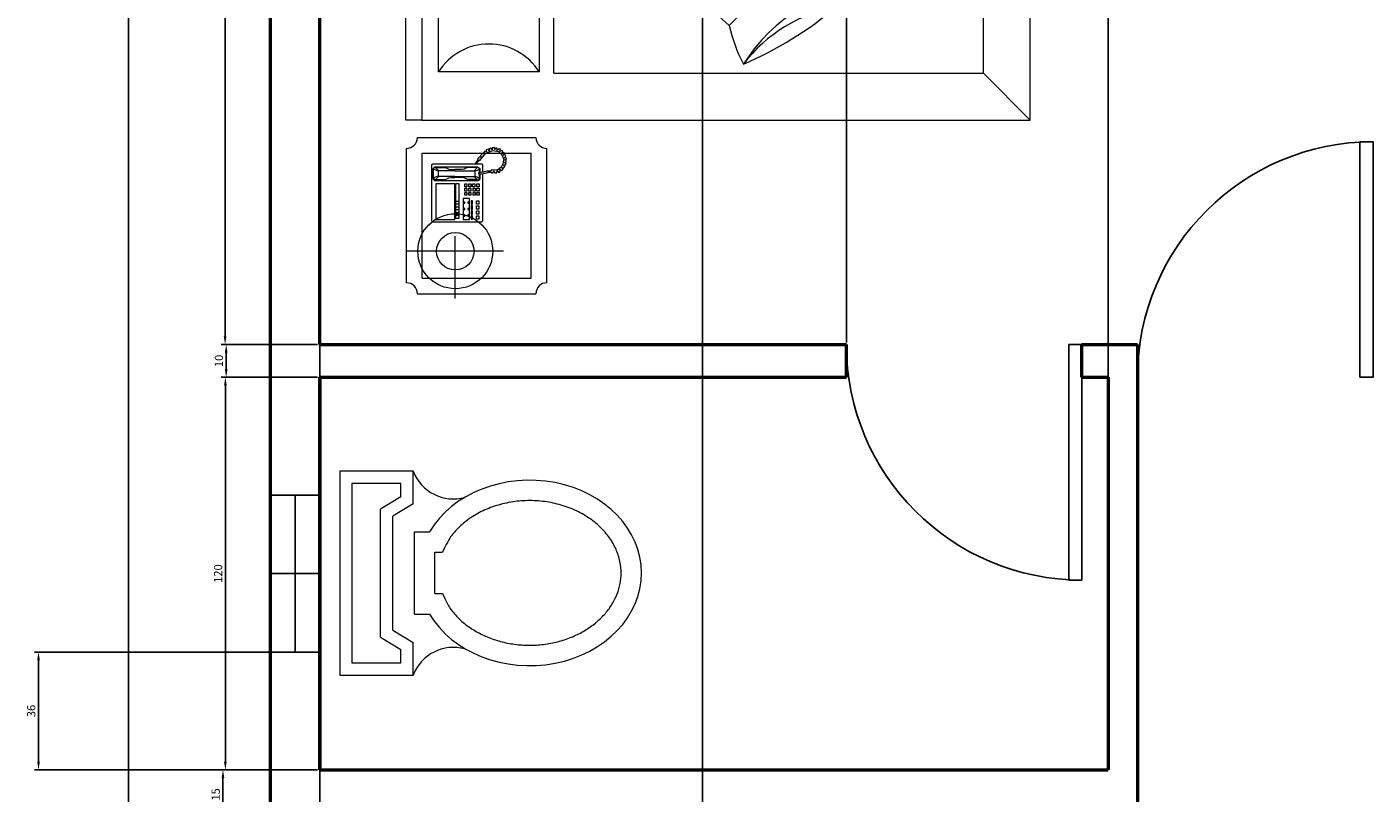
# Model space of a CAD drawing. Units: inches. Extents: x 604 to 3492, y -123 to 1737.
# Tile 13 of 20: x 1500 to 1912, y 836 to 1070. Entities that reach past the tile are written whole.
import ezdxf

# ---------------------------------------------------------------- set-up
doc = ezdxf.new("R2010")
doc.units = ezdxf.units.IN
for name, color, linetype, lineweight in [('A-ANNO-DIMS', 2, 'Continuous', 18), ('A-DOOR', 3, 'Continuous', 25), ('A-FLOR-FIXT', 9, 'Continuous', 18), ('A-FURN', 8, 'Continuous', 18), ('A-GLAZ', 4, 'Continuous', 25), ('A-WALL', 7, 'Continuous', 50)]:
    doc.layers.add(name, color=color, linetype=linetype, lineweight=lineweight)
doc.styles.get("Standard").update_dxf_attribs({"font": 'arial.ttf'})
doc.dimstyles.new('ISO-25', dxfattribs={"dimtxt": 2.5, "dimasz": 2.5, "dimexe": 1.25, "dimexo": 0.625, "dimtad": 1, "dimtxsty": 'Standard', "dimcen": 2.5, "dimadec": 0, "dimazin": 0, "dimtfac": 1, "dimtmove": 0, "dimatfit": 3, "dimfxl": 1, "dimarcsym": 0})

# ---------------------------------------------------------------- blocks, each defined once
blk = doc.blocks.new('A$C50B66110')
for p, q in [((0.0503, 1.9981), (0.4803, 1.9981)), ((0.1513, 1.6871), (0.1513, 1.9967)), ((0.5716, 1.9488), (0.5716, 2)), ((0.5716, 2), (2.0719, 2)), ((2.0719, 1.9488), (2.0719, 2)), ((2.5701, 1.9993), (2.1401, 1.9993)), ((0.0153, 1.9631), (0.0153, 1.5831)), ((0.0653, 1.9481), (0.0653, 1.5981)), ((0.0653, 1.9481), (0.4653, 1.9481)), ((0.4653, 1.9481), (0.4653, 1.5981)), ((0.5153, 1.9631), (0.5153, 1.5831)), ((2.0719, 1.9488), (0.5716, 1.9488)), ((0.5716, 1.9488), (0.5716, 0)), ((2.0719, 0), (2.0719, 1.9488)), ((2.1051, 1.9643), (2.1051, 1.5843)), ((2.1551, 1.9493), (2.1551, 1.5993)), ((2.5551, 1.9493), (2.1551, 1.9493)), ((2.5551, 1.9493), (2.5551, 1.5993)), ((2.6051, 1.9643), (2.6051, 1.5843)), ((2.3505, 1.62), (2.3505, 1.9295)), ((0.7257, 1.5725), (0.7257, 1.8954)), ((0.7257, 1.8954), (1.2113, 1.8954)), ((1.2113, 1.8954), (1.2113, 1.5725)), ((1.4007, 1.5725), (1.4007, 1.8954)), ((1.4007, 1.8954), (1.8863, 1.8954)), ((1.8863, 1.8954), (1.8863, 1.5725)), ((0, 1.8416), (0.2001, 1.8416)), ((2.5018, 1.7744), (2.2017, 1.7744)), ((0.0653, 1.5981), (0.4653, 1.5981)), ((2.5551, 1.5993), (2.1551, 1.5993)), ((1.2113, 1.5725), (0.7257, 1.5725)), ((1.8863, 1.5725), (1.4007, 1.5725)), ((0.0503, 1.5481), (0.4803, 1.5481)), ((1.5665, 1.5254), (1.5665, 1.0802)), ((1.5665, 1.5254), (1.9219, 1.0802)), ((2.5701, 1.5493), (2.1401, 1.5493)), ((1.9219, 1.0802), (1.5665, 1.0802)), ((0.5716, 0), (0.7216, 0.15)), ((2.0719, 0), (1.9219, 0.15)), ((0.5716, 0), (2.0719, 0))]:
    blk.add_line(p, q)
at = {"linetype": 'ByBlock'}
for p, q in [((0.2481, 1.9162), (0.2458, 1.9139)), ((0.2458, 1.9139), (0.2458, 1.7562)), ((0.2481, 1.9162), (0.4287, 1.9162)), ((0.2526, 1.9036), (0.2526, 1.8431)), ((0.3669, 1.9036), (0.2526, 1.9036)), ((0.3669, 1.8431), (0.3669, 1.9036)), ((0.3772, 1.9071), (0.3818, 1.9128)), ((0.3772, 1.7688), (0.3772, 1.9071)), ((0.3818, 1.9094), (0.3807, 1.9048)), ((0.3807, 1.9048), (0.3807, 1.8739)), ((0.3807, 1.9048), (0.3909, 1.8945)), ((0.3818, 1.9128), (0.4161, 1.9128)), ((0.3864, 1.9116), (0.3818, 1.9094)), ((0.3921, 1.8968), (0.3864, 1.9116)), ((0.3864, 1.9116), (0.4138, 1.9116)), ((0.4081, 1.8968), (0.4138, 1.9116)), ((0.4195, 1.9048), (0.4092, 1.8945)), ((0.4138, 1.9116), (0.4184, 1.9094)), ((0.4161, 1.9128), (0.4218, 1.9071)), ((0.4184, 1.9094), (0.4195, 1.9048)), ((0.4195, 1.9048), (0.4195, 1.8739)), ((0.4218, 1.9071), (0.4218, 1.7699)), ((0.4287, 1.9162), (0.4309, 1.9139)), ((0.4309, 1.9139), (0.4309, 1.7562)), ((0.3807, 1.8739), (0.3829, 1.8682)), ((0.3829, 1.8682), (0.3864, 1.8625)), ((0.3864, 1.8625), (0.3875, 1.8545)), ((0.3875, 1.8545), (0.3875, 1.8431)), ((0.3909, 1.8945), (0.3921, 1.8968)), ((0.3909, 1.8431), (0.3909, 1.8945)), ((0.4081, 1.8968), (0.3921, 1.8968)), ((0.4092, 1.8945), (0.4081, 1.8968)), ((0.4092, 1.8431), (0.4092, 1.8945)), ((0.4138, 1.8625), (0.4127, 1.8545)), ((0.4127, 1.8545), (0.4127, 1.8431)), ((0.4172, 1.8682), (0.4138, 1.8625)), ((0.4195, 1.8739), (0.4172, 1.8682)), ((0.2526, 1.8431), (0.3669, 1.8431)), ((0.3201, 1.8168), (0.2526, 1.8168)), ((0.2526, 1.8168), (0.2526, 1.7962)), ((0.2572, 1.8408), (0.2572, 1.8294)), ((0.3669, 1.8408), (0.2572, 1.8408)), ((0.2572, 1.8294), (0.3669, 1.8294)), ((0.2675, 1.8145), (0.2641, 1.8145)), ((0.2641, 1.8145), (0.2641, 1.8111)), ((0.2641, 1.8111), (0.2675, 1.8111)), ((0.2664, 1.8408), (0.2664, 1.8294)), ((0.2675, 1.8111), (0.2675, 1.8145)), ((0.2755, 1.8408), (0.2755, 1.8294)), ((0.2846, 1.8408), (0.2846, 1.8294)), ((0.2846, 1.8145), (0.2846, 1.8111)), ((0.2881, 1.8145), (0.2846, 1.8145)), ((0.2846, 1.8111), (0.2881, 1.8111)), ((0.2881, 1.8111), (0.2881, 1.8145)), ((0.2938, 1.8408), (0.2938, 1.8294)), ((0.3029, 1.8408), (0.3029, 1.8294)), ((0.3052, 1.8145), (0.3052, 1.8111)), ((0.3086, 1.8145), (0.3052, 1.8145)), ((0.3052, 1.8111), (0.3086, 1.8111)), ((0.3086, 1.8111), (0.3086, 1.8145)), ((0.3121, 1.8408), (0.3121, 1.8294)), ((0.3201, 1.7962), (0.3201, 1.8168)), ((0.3304, 1.8111), (0.3395, 1.8111)), ((0.3304, 1.8042), (0.3304, 1.8111)), ((0.3395, 1.8111), (0.3395, 1.8042)), ((0.3441, 1.8042), (0.3441, 1.8111)), ((0.3441, 1.8111), (0.3532, 1.8111)), ((0.3532, 1.8111), (0.3532, 1.8042)), ((0.3578, 1.8111), (0.3669, 1.8111)), ((0.3578, 1.8042), (0.3578, 1.8111)), ((0.3669, 1.8294), (0.3669, 1.8408)), ((0.3669, 1.8111), (0.3669, 1.8042)), ((0.3829, 1.8076), (0.3864, 1.8134)), ((0.3864, 1.8134), (0.3875, 1.8214)), ((0.3875, 1.8214), (0.3875, 1.8431)), ((0.3909, 1.8431), (0.3909, 1.7813)), ((0.4092, 1.8431), (0.4092, 1.7813)), ((0.4127, 1.8214), (0.4127, 1.8431)), ((0.4138, 1.8134), (0.4127, 1.8214)), ((0.4172, 1.8076), (0.4138, 1.8134)), ((0.2526, 1.7962), (0.3201, 1.7962)), ((0.2652, 1.7905), (0.2538, 1.7905)), ((0.2538, 1.7905), (0.2538, 1.7859)), ((0.2538, 1.7859), (0.2652, 1.7859)), ((0.2538, 1.7665), (0.2538, 1.7733)), ((0.2538, 1.7733), (0.2652, 1.7733)), ((0.2641, 1.8019), (0.2641, 1.7985)), ((0.2675, 1.8019), (0.2641, 1.8019)), ((0.2641, 1.7985), (0.2675, 1.7985)), ((0.2652, 1.7859), (0.2652, 1.7905)), ((0.2652, 1.7733), (0.2652, 1.7665)), ((0.2675, 1.7985), (0.2675, 1.8019)), ((0.2812, 1.7905), (0.2698, 1.7905)), ((0.2698, 1.7905), (0.2698, 1.7859)), ((0.2698, 1.7859), (0.2812, 1.7859)), ((0.2698, 1.7665), (0.2698, 1.7733)), ((0.2698, 1.7733), (0.2812, 1.7733)), ((0.2812, 1.7859), (0.2812, 1.7905)), ((0.2812, 1.7733), (0.2812, 1.7665)), ((0.2846, 1.8019), (0.2846, 1.7985)), ((0.2881, 1.8019), (0.2846, 1.8019)), ((0.2846, 1.7985), (0.2881, 1.7985)), ((0.2972, 1.7905), (0.2858, 1.7905)), ((0.2858, 1.7905), (0.2858, 1.7859)), ((0.2858, 1.7859), (0.2972, 1.7859)), ((0.2858, 1.7665), (0.2858, 1.7733)), ((0.2858, 1.7733), (0.2972, 1.7733)), ((0.2881, 1.7985), (0.2881, 1.8019)), ((0.2972, 1.7859), (0.2972, 1.7905)), ((0.2972, 1.7733), (0.2972, 1.7665)), ((0.3018, 1.7905), (0.3018, 1.7859)), ((0.3132, 1.7905), (0.3018, 1.7905)), ((0.3018, 1.7859), (0.3132, 1.7859)), ((0.3018, 1.7733), (0.3132, 1.7733)), ((0.3018, 1.7665), (0.3018, 1.7733)), ((0.3052, 1.8019), (0.3052, 1.7985)), ((0.3086, 1.8019), (0.3052, 1.8019)), ((0.3052, 1.7985), (0.3086, 1.7985)), ((0.3086, 1.7985), (0.3086, 1.8019)), ((0.3132, 1.7859), (0.3132, 1.7905)), ((0.3132, 1.7733), (0.3132, 1.7665)), ((0.3395, 1.8042), (0.3304, 1.8042)), ((0.3304, 1.7985), (0.3395, 1.7985)), ((0.3304, 1.7916), (0.3304, 1.7985)), ((0.3395, 1.7916), (0.3304, 1.7916)), ((0.3304, 1.7779), (0.3304, 1.7848)), ((0.3304, 1.7848), (0.3395, 1.7848)), ((0.3395, 1.7779), (0.3304, 1.7779)), ((0.3304, 1.7722), (0.3395, 1.7722)), ((0.3304, 1.7653), (0.3304, 1.7722)), ((0.3395, 1.7985), (0.3395, 1.7916)), ((0.3395, 1.7848), (0.3395, 1.7779)), ((0.3395, 1.7722), (0.3395, 1.7653)), ((0.3532, 1.8042), (0.3441, 1.8042)), ((0.3441, 1.7985), (0.3532, 1.7985)), ((0.3441, 1.7916), (0.3441, 1.7985)), ((0.3532, 1.7916), (0.3441, 1.7916)), ((0.3441, 1.7779), (0.3441, 1.7848)), ((0.3441, 1.7848), (0.3532, 1.7848)), ((0.3532, 1.7779), (0.3441, 1.7779)), ((0.3441, 1.7722), (0.3532, 1.7722)), ((0.3441, 1.7653), (0.3441, 1.7722)), ((0.3532, 1.7985), (0.3532, 1.7916)), ((0.3532, 1.7848), (0.3532, 1.7779)), ((0.3532, 1.7722), (0.3532, 1.7653)), ((0.3669, 1.8042), (0.3578, 1.8042)), ((0.3578, 1.7985), (0.3669, 1.7985)), ((0.3578, 1.7916), (0.3578, 1.7985)), ((0.3669, 1.7916), (0.3578, 1.7916)), ((0.3578, 1.7791), (0.3578, 1.7859)), ((0.3578, 1.7859), (0.3669, 1.7859)), ((0.3669, 1.7791), (0.3578, 1.7791)), ((0.3578, 1.7653), (0.3578, 1.7722)), ((0.3578, 1.7722), (0.3669, 1.7722)), ((0.3669, 1.7985), (0.3669, 1.7916)), ((0.3669, 1.7859), (0.3669, 1.7791)), ((0.3669, 1.7722), (0.3669, 1.7653)), ((0.3829, 1.7631), (0.3772, 1.7688)), ((0.3807, 1.8019), (0.3829, 1.8076)), ((0.3807, 1.7711), (0.3807, 1.8019)), ((0.3807, 1.7711), (0.3909, 1.7813)), ((0.3818, 1.7665), (0.3807, 1.7711)), ((0.3921, 1.7791), (0.3864, 1.7642)), ((0.3909, 1.7813), (0.3921, 1.7791)), ((0.4081, 1.7791), (0.3921, 1.7791)), ((0.4092, 1.7813), (0.4081, 1.7791)), ((0.4081, 1.7791), (0.4138, 1.7642)), ((0.4195, 1.7711), (0.4092, 1.7813)), ((0.4218, 1.7699), (0.4161, 1.7631)), ((0.4195, 1.8019), (0.4172, 1.8076)), ((0.4184, 1.7665), (0.4195, 1.7711)), ((0.4195, 1.7711), (0.4195, 1.8019)), ((0.4378, 1.7742), (0.4309, 1.7768)), ((0.4309, 1.7722), (0.436, 1.7708)), ((0.436, 1.7708), (0.4406, 1.7672)), ((0.441, 1.771), (0.4378, 1.7742)), ((0.4434, 1.7688), (0.441, 1.771)), ((0.4477, 1.7704), (0.4434, 1.7688)), ((0.4497, 1.7684), (0.4477, 1.7704)), ((0.4481, 1.765), (0.4497, 1.7684)), ((0.2458, 1.7562), (0.2481, 1.7539)), ((0.4, 1.7539), (0.2481, 1.7539)), ((0.2652, 1.7665), (0.2538, 1.7665)), ((0.2812, 1.7665), (0.2698, 1.7665)), ((0.2972, 1.7665), (0.2858, 1.7665)), ((0.3132, 1.7665), (0.3018, 1.7665)), ((0.3395, 1.7653), (0.3304, 1.7653)), ((0.3532, 1.7653), (0.3441, 1.7653)), ((0.3669, 1.7653), (0.3578, 1.7653)), ((0.3864, 1.7642), (0.3818, 1.7665)), ((0.399, 1.7631), (0.3829, 1.7631)), ((0.3864, 1.7642), (0.399, 1.7642)), ((0.4024, 1.7676), (0.3989, 1.7676)), ((0.3989, 1.7676), (0.3991, 1.7578)), ((0.3991, 1.7578), (0.4019, 1.7462)), ((0.4019, 1.7462), (0.4047, 1.7353)), ((0.4026, 1.7254), (0.4021, 1.7198)), ((0.403, 1.7585), (0.4024, 1.7676)), ((0.4026, 1.7642), (0.4138, 1.7642)), ((0.4051, 1.7279), (0.4026, 1.7254)), ((0.4161, 1.7631), (0.4027, 1.7631)), ((0.4047, 1.7511), (0.403, 1.7585)), ((0.4287, 1.7539), (0.404, 1.7539)), ((0.4047, 1.7353), (0.4044, 1.7293)), ((0.4044, 1.7293), (0.4051, 1.7279)), ((0.4074, 1.7402), (0.4047, 1.7511)), ((0.4081, 1.7346), (0.4074, 1.7402)), ((0.4079, 1.7286), (0.4081, 1.7346)), ((0.4121, 1.7256), (0.4079, 1.7286)), ((0.4111, 1.7203), (0.4121, 1.7256)), ((0.4138, 1.7642), (0.4184, 1.7665)), ((0.4309, 1.7562), (0.4287, 1.7539)), ((0.4406, 1.7672), (0.4418, 1.7656)), ((0.4443, 1.7658), (0.4418, 1.7633)), ((0.4418, 1.7656), (0.4443, 1.7658)), ((0.4418, 1.7633), (0.4511, 1.7551)), ((0.4509, 1.7672), (0.4481, 1.765)), ((0.4539, 1.764), (0.4509, 1.7672)), ((0.4511, 1.7551), (0.4662, 1.7422)), ((0.4515, 1.7573), (0.4539, 1.764)), ((0.4577, 1.7605), (0.4515, 1.7573)), ((0.463, 1.7555), (0.4577, 1.7605)), ((0.4618, 1.7482), (0.463, 1.7555)), ((0.467, 1.7515), (0.4618, 1.7482)), ((0.4664, 1.7418), (0.4741, 1.72)), ((0.4714, 1.7468), (0.467, 1.7515)), ((0.4696, 1.7418), (0.4714, 1.7468)), ((0.4766, 1.7425), (0.4697, 1.7418)), ((0.472, 1.733), (0.4787, 1.7356)), ((0.4794, 1.7332), (0.472, 1.733)), ((0.4761, 1.7233), (0.481, 1.7279)), ((0.4787, 1.7356), (0.4766, 1.7425)), ((0.481, 1.7279), (0.4794, 1.7332)), ((0.4021, 1.7198), (0.4088, 1.7187)), ((0.4088, 1.7187), (0.4023, 1.7147)), ((0.4023, 1.7147), (0.4028, 1.7085)), ((0.4028, 1.7085), (0.4102, 1.7078)), ((0.4102, 1.7078), (0.4037, 1.7027)), ((0.4037, 1.7027), (0.4067, 1.6974)), ((0.4067, 1.6974), (0.4137, 1.6988)), ((0.4137, 1.6988), (0.4104, 1.6923)), ((0.4104, 1.6923), (0.4139, 1.6881)), ((0.4123, 1.7057), (0.4111, 1.7203)), ((0.4211, 1.6946), (0.4123, 1.7057)), ((0.4139, 1.6881), (0.4192, 1.692)), ((0.4192, 1.692), (0.4183, 1.6858)), ((0.4183, 1.6858), (0.4227, 1.683)), ((0.4333, 1.6881), (0.4211, 1.6946)), ((0.4227, 1.683), (0.4283, 1.6876)), ((0.4283, 1.6876), (0.4276, 1.68)), ((0.4324, 1.6786), (0.4354, 1.6849)), ((0.4472, 1.6869), (0.4333, 1.6881)), ((0.4354, 1.6849), (0.4382, 1.6786)), ((0.4421, 1.6782), (0.4437, 1.6849)), ((0.4437, 1.6849), (0.4463, 1.6775)), ((0.4606, 1.6927), (0.4472, 1.6869)), ((0.4507, 1.6786), (0.4509, 1.6849)), ((0.4509, 1.6849), (0.4562, 1.6802)), ((0.4562, 1.6802), (0.4599, 1.6821)), ((0.4592, 1.689), (0.4641, 1.683)), ((0.4599, 1.6821), (0.4592, 1.689)), ((0.4708, 1.7027), (0.4606, 1.6927)), ((0.4641, 1.683), (0.4678, 1.6863)), ((0.465, 1.6925), (0.4715, 1.6897)), ((0.4678, 1.6863), (0.465, 1.6925)), ((0.4741, 1.72), (0.4708, 1.7027)), ((0.4745, 1.6925), (0.4713, 1.6988)), ((0.4713, 1.6988), (0.478, 1.6967)), ((0.4715, 1.6897), (0.4745, 1.6925)), ((0.4743, 1.7075), (0.4815, 1.7073)), ((0.4798, 1.7013), (0.4743, 1.7075)), ((0.4824, 1.7233), (0.4761, 1.7233)), ((0.4764, 1.7154), (0.4835, 1.7175)), ((0.4824, 1.7119), (0.4764, 1.7154)), ((0.478, 1.6967), (0.4798, 1.7013)), ((0.4815, 1.7073), (0.4824, 1.7119)), ((0.4835, 1.7175), (0.4824, 1.7233)), ((0.4276, 1.68), (0.4324, 1.6786)), ((0.4382, 1.6786), (0.4421, 1.6782)), ((0.4463, 1.6775), (0.4507, 1.6786)), ((0.7216, 1.5254), (1.9219, 1.5254)), ((0.7216, 1.5254), (0.7216, 0.15)), ((1.9219, 0.15), (1.9219, 1.5254)), ((0.7216, 0.15), (1.9219, 0.15))]:
    blk.add_line(p, q, dxfattribs=at)
for centre, radius in [((0.1513, 1.8416), 0.12), ((0.1513, 1.8416), 0.06), ((2.3505, 1.7744), 0.12), ((2.3505, 1.7744), 0.06)]:
    blk.add_circle(centre, radius)
for centre, radius, start, end in [((0.0153, 1.9981), 0.035, 270, 0), ((0.5153, 1.9981), 0.035, 180, 270), ((2.1051, 1.9993), 0.035, 270, 0), ((2.6051, 1.9993), 0.035, 180, 270), ((0.6244, 1.734), 0.1906, 302.1202, 57.8798), ((1.3126, 1.734), 0.1906, 122.1202, 237.8798), ((1.2994, 1.734), 0.1906, 302.1202, 57.8798), ((1.9876, 1.734), 0.1906, 122.1202, 237.8798), ((0.0153, 1.5481), 0.035, 0, 90), ((0.5153, 1.5481), 0.035, 90, 180), ((2.1051, 1.5493), 0.035, 0, 90), ((2.6051, 1.5493), 0.035, 90, 180), ((1.1502, 0.7366), 0.3575, 102.4782, 140.4625), ((0.328, 0.4368), 0.9879, 28.4971, 41.0566), ((1.9117, 1.3157), 0.8697, 195.336, 226.4193), ((0.9996, 0.4307), 0.548, 103.2034, 117.0362), ((1.656, 1.7093), 1.0798, 223.6306, 251.4288), ((0.4482, 0.4408), 0.5655, 5.3391, 57.6895), ((1.8226, 1.3753), 1.1652, 203.0642, 220.3209), ((0.4548, 0.5307), 0.4879, 10.6986, 52.6864), ((0.5648, 0.4378), 0.7874, 18.3527, 36.6851), ((1.4166, 0.4903), 0.3575, 154.0418, 192.0262), ((1.1403, -0.3401), 0.9879, 80.0607, 92.6202), ((-0.0179, 2.4352), 2.1977, 305.2966, 307.2418), ((1.5981, 0.9345), 0.734, 205.259, 216.9351), ((1.3672, 0.0075), 0.6085, 71.81, 120.1351), ((1.2867, -0.154), 0.7874, 69.9163, 88.2487), ((1.4431, 0.1219), 0.4774, 76.1849, 142.0017), ((-0.6401, 0.6314), 2.1977, 349.4884, 358.8054), ((-0.0179, 2.4352), 2.1977, 297.9248, 299.3793), ((1.5626, 0.1822), 0.548, 154.767, 168.5998), ((1.2678, 0.9611), 0.6885, 250.2936, 293.6414), ((1.3343, 1.4141), 1.1652, 254.6278, 271.8845), ((1.5399, 0.9642), 0.734, 256.8226, 268.4988)]:
    blk.add_arc(centre, radius, start, end)
blk = doc.blocks.new('A$C7C8779AE')
for p, q in [((0, 0.7405), (0, 0.5605)), ((0.5, 0.7405), (0, 0.7405)), ((0.5, 0.5605), (0.5, 0.7405)), ((0.47, 0.7105), (0.03, 0.7105)), ((0.03, 0.7105), (0.03, 0.5905)), ((0.47, 0.5905), (0.47, 0.7105)), ((0.093, 0.6405), (0.063, 0.5905)), ((0.093, 0.6405), (0.407, 0.6405)), ((0.437, 0.5905), (0.407, 0.6405)), ((0.11, 0.6105), (0.08, 0.5605)), ((0.11, 0.6105), (0.39, 0.6105)), ((0.42, 0.5605), (0.39, 0.6105)), ((0.03, 0.5905), (0.063, 0.5905)), ((0.437, 0.5905), (0.47, 0.5905)), ((0, 0.5605), (0.08, 0.5605)), ((0.1497, 0.557), (0.1497, 0.5203)), ((0.1497, 0.557), (0.3514, 0.557)), ((0.3514, 0.557), (0.3514, 0.5203)), ((0.42, 0.5605), (0.5, 0.5605)), ((0.1997, 0.507), (0.1997, 0.4879)), ((0.1997, 0.507), (0.3014, 0.507)), ((0.3014, 0.507), (0.3014, 0.4879))]:
    blk.add_line(p, q)
for centre, start, end in [((-0.0386, 0.4613), 344.642, 68.7339), ((0.5386, 0.4613), 111.2661, 195.358)]:
    blk.add_arc(centre, 0.1064, start, end)
blk.add_ellipse((0.2506, 0.2744), major_axis=(0, 0.2744), ratio=0.828948, start_param=0.459479, end_param=5.823706)
blk.add_open_spline([(0.1997, 0.4879), (0.1697, 0.474), (0.1642, 0.4702), (0.1512, 0.4602), (0.1438, 0.4535), (0.1298, 0.4388), (0.1233, 0.4306), (0.1111, 0.4131), (0.1055, 0.4037), (0.0956, 0.3838), (0.0912, 0.3733), (0.0838, 0.3516), (0.0808, 0.3403), (0.0762, 0.3172), (0.0746, 0.3055), (0.073, 0.2817), (0.0729, 0.2698), (0.0743, 0.246), (0.0758, 0.2342), (0.0801, 0.2111), (0.0831, 0.1998), (0.0903, 0.1779), (0.0945, 0.1673), (0.1043, 0.1473), (0.1098, 0.1378), (0.1218, 0.12), (0.1283, 0.1118), (0.1421, 0.0968), (0.1494, 0.09), (0.1646, 0.078), (0.1725, 0.0728), (0.1887, 0.064), (0.1969, 0.0603), (0.2137, 0.0547), (0.2222, 0.0527), (0.2392, 0.0502), (0.2478, 0.0498), (0.2664, 0.0505), (0.2764, 0.052), (0.2963, 0.0573), (0.3061, 0.061), (0.3253, 0.0707), (0.3346, 0.0766), (0.3525, 0.0906), (0.3611, 0.0987), (0.3771, 0.1169), (0.3845, 0.127), (0.3978, 0.1488), (0.4037, 0.1605), (0.4137, 0.1853), (0.4178, 0.1983), (0.424, 0.2251), (0.4261, 0.2389), (0.4282, 0.2668), (0.4283, 0.2809), (0.4262, 0.3088), (0.4241, 0.3226), (0.418, 0.3495), (0.414, 0.3625), (0.404, 0.3873), (0.3982, 0.3991), (0.385, 0.421), (0.3776, 0.4311), (0.3617, 0.4494), (0.3531, 0.4575), (0.3382, 0.4693), (0.3321, 0.4736), (0.3014, 0.4879)], degree=3, knots=[0.459479, 0.459479, 0.459479, 0.459479, 0.567422, 0.567422, 0.720865, 0.720865, 0.874307, 0.874307, 1.02775, 1.02775, 1.181192, 1.181192, 1.334635, 1.334635, 1.488077, 1.488077, 1.64152, 1.64152, 1.794963, 1.794963, 1.948405, 1.948405, 2.101848, 2.101848, 2.25529, 2.25529, 2.408733, 2.408733, 2.562175, 2.562175, 2.715618, 2.715618, 2.86906, 2.86906, 3.022503, 3.022503, 3.175946, 3.175946, 3.356457, 3.356457, 3.536968, 3.536968, 3.717479, 3.717479, 3.89799, 3.89799, 4.078501, 4.078501, 4.259012, 4.259012, 4.439523, 4.439523, 4.620035, 4.620035, 4.800546, 4.800546, 4.981057, 4.981057, 5.161568, 5.161568, 5.342079, 5.342079, 5.52259, 5.52259, 5.703101, 5.703101, 5.823706, 5.823706, 5.823706, 5.823706])
blk = doc.blocks.new('*D61')
at = {"layer": 'A-ANNO-DIMS', "color": 0, "lineweight": -2, "transparency": 16777216}
for p, q in [((1588.95, 1272.7), (1559.41, 1272.7)), ((1560.66, 1270.2), (1560.66, 975.2)), ((1588.95, 972.7), (1559.41, 972.7))]:
    blk.add_line(p, q, dxfattribs=at)
at = {"layer": 'A-ANNO-DIMS', "color": 0, "transparency": 16777216}
for points in [[(1560.24, 1270.2), (1561.07, 1270.2), (1560.66, 1272.7)], [(1560.24, 975.2), (1561.07, 975.2), (1560.66, 972.7)]]:
    blk.add_solid(points, dxfattribs=at)
at = {"layer": 'Defpoints', "color": 0, "transparency": 16777216}
for p in [(1589.57, 1272.7), (1560.66, 972.7), (1589.57, 972.7)]:
    blk.add_point(p, dxfattribs=at)
at = {"layer": 'A-ANNO-DIMS', "color": 0, "transparency": 16777216, "insert": (1558.76, 1122.7), "char_height": 2.5, "attachment_point": 5, "rotation": 90}
blk.add_mtext('300', dxfattribs=at)
blk = doc.blocks.new('*D62')
at = {"layer": 'A-ANNO-DIMS', "color": 0, "lineweight": -2, "transparency": 16777216}
for p, q in [((1588.95, 972.7), (1559.74, 972.7)), ((1560.99, 970.2), (1560.99, 965.2)), ((1588.95, 962.7), (1559.74, 962.7))]:
    blk.add_line(p, q, dxfattribs=at)
at = {"layer": 'A-ANNO-DIMS', "color": 0, "transparency": 16777216}
for points in [[(1560.57, 970.2), (1561.41, 970.2), (1560.99, 972.7)], [(1560.57, 965.2), (1561.41, 965.2), (1560.99, 962.7)]]:
    blk.add_solid(points, dxfattribs=at)
at = {"layer": 'Defpoints', "color": 0, "transparency": 16777216}
for p in [(1589.57, 972.7), (1560.99, 962.7), (1589.57, 962.7)]:
    blk.add_point(p, dxfattribs=at)
at = {"layer": 'A-ANNO-DIMS', "color": 0, "transparency": 16777216, "insert": (1559.09, 967.7), "char_height": 2.5, "attachment_point": 5, "rotation": 90}
blk.add_mtext('10', dxfattribs=at)
blk = doc.blocks.new('*D63')
at = {"layer": 'A-ANNO-DIMS', "color": 0, "lineweight": -2, "transparency": 16777216}
for p, q in [((1588.95, 962.7), (1559.49, 962.7)), ((1560.74, 960.2), (1560.74, 845.2)), ((1588.95, 842.7), (1559.49, 842.7))]:
    blk.add_line(p, q, dxfattribs=at)
at = {"layer": 'A-ANNO-DIMS', "color": 0, "transparency": 16777216}
for points in [[(1560.33, 960.2), (1561.16, 960.2), (1560.74, 962.7)], [(1560.33, 845.2), (1561.16, 845.2), (1560.74, 842.7)]]:
    blk.add_solid(points, dxfattribs=at)
at = {"layer": 'Defpoints', "color": 0, "transparency": 16777216}
for p in [(1589.57, 962.7), (1560.74, 842.7), (1589.57, 842.7)]:
    blk.add_point(p, dxfattribs=at)
at = {"layer": 'A-ANNO-DIMS', "color": 0, "transparency": 16777216, "insert": (1558.84, 902.7), "char_height": 2.5, "attachment_point": 5, "rotation": 90}
blk.add_mtext('120', dxfattribs=at)
blk = doc.blocks.new('*D64')
at = {"layer": 'A-ANNO-DIMS', "color": 0, "lineweight": -2, "transparency": 16777216}
for p, q in [((1588.95, 842.7), (1558.76, 842.7)), ((1560.01, 840.2), (1560.01, 830.2)), ((1588.95, 827.7), (1558.76, 827.7))]:
    blk.add_line(p, q, dxfattribs=at)
at = {"layer": 'A-ANNO-DIMS', "color": 0, "transparency": 16777216}
for points in [[(1559.6, 840.2), (1560.43, 840.2), (1560.01, 842.7)], [(1559.6, 830.2), (1560.43, 830.2), (1560.01, 827.7)]]:
    blk.add_solid(points, dxfattribs=at)
at = {"layer": 'Defpoints', "color": 0, "transparency": 16777216}
for p in [(1589.57, 842.7), (1560.01, 827.7), (1589.57, 827.7)]:
    blk.add_point(p, dxfattribs=at)
at = {"layer": 'A-ANNO-DIMS', "color": 0, "transparency": 16777216, "insert": (1558.11, 835.2), "char_height": 2.5, "attachment_point": 5, "rotation": 90}
blk.add_mtext('15', dxfattribs=at)
blk = doc.blocks.new('*D69')
at = {"layer": 'A-ANNO-DIMS', "color": 0, "lineweight": -2, "transparency": 16777216}
for p, q in [((1573.95, 1287.7), (1529.86, 1287.7)), ((1531.11, 290.2), (1531.11, 1285.2)), ((1573.95, 287.7), (1529.86, 287.7))]:
    blk.add_line(p, q, dxfattribs=at)
at = {"layer": 'A-ANNO-DIMS', "color": 0, "transparency": 16777216}
for points in [[(1530.69, 1285.2), (1531.52, 1285.2), (1531.11, 1287.7)], [(1530.69, 290.2), (1531.52, 290.2), (1531.11, 287.7)]]:
    blk.add_solid(points, dxfattribs=at)
at = {"layer": 'Defpoints', "color": 0, "transparency": 16777216}
for p in [(1531.11, 1287.7), (1574.57, 1287.7), (1574.57, 287.7)]:
    blk.add_point(p, dxfattribs=at)
at = {"layer": 'A-ANNO-DIMS', "color": 0, "transparency": 16777216, "insert": (1529.21, 787.7), "char_height": 2.5, "attachment_point": 5, "rotation": 90}
blk.add_mtext('1000', dxfattribs=at)
blk = doc.blocks.new('DOOR-SWING-72')
for p, q in [((0, 72), (0, 0)), ((0, 0), (4, 0)), ((0, 0), (4, 0))]:
    blk.add_line(p, q)
blk.add_lwpolyline([(0, 72), (0, 0), (4, 0), (4, 72)], close=True)
blk.add_arc((0, 0), 72, 0, 90)
blk = doc.blocks.new('WIN-48')
for p, q in [((0, 48), (15, 48)), ((7.5, 48), (7.5, 0)), ((15, 48), (15, 0)), ((0, 24), (15, 24))]:
    blk.add_line(p, q)
blk.add_lwpolyline([(15, 0), (0, 0), (0, 48), (15, 48)], close=True)
blk = doc.blocks.new('*D100')
at = {"layer": 'A-ANNO-DIMS', "color": 0, "lineweight": -2, "transparency": 16777216}
for p, q in [((1589.57, 843.33), (1589.57, 1359.9)), ((1592.07, 1358.65), (1828.07, 1358.65)), ((1830.57, 843.33), (1830.57, 1359.9))]:
    blk.add_line(p, q, dxfattribs=at)
at = {"layer": 'A-ANNO-DIMS', "color": 0, "transparency": 16777216}
for points in [[(1592.07, 1359.07), (1592.07, 1358.23), (1589.57, 1358.65)], [(1828.07, 1359.07), (1828.07, 1358.23), (1830.57, 1358.65)]]:
    blk.add_solid(points, dxfattribs=at)
at = {"layer": 'Defpoints', "color": 0, "transparency": 16777216}
for p in [(1830.57, 1358.65), (1589.57, 842.7), (1830.57, 842.7)]:
    blk.add_point(p, dxfattribs=at)
at = {"layer": 'A-ANNO-DIMS', "color": 0, "transparency": 16777216, "insert": (1710.07, 1360.53), "char_height": 2.5, "attachment_point": 5}
blk.add_mtext('241', dxfattribs=at)
blk = doc.blocks.new('*D102')
at = {"layer": 'A-ANNO-DIMS', "color": 0, "lineweight": -2, "transparency": 16777216}
for p, q in [((1839.57, 972.08), (1839.57, 215.5)), ((2023.07, 972.08), (2023.07, 215.5)), ((1842.07, 216.75), (2020.57, 216.75))]:
    blk.add_line(p, q, dxfattribs=at)
at = {"layer": 'A-ANNO-DIMS', "color": 0, "transparency": 16777216}
for points in [[(1842.07, 217.17), (1842.07, 216.33), (1839.57, 216.75)], [(2020.57, 217.17), (2020.57, 216.33), (2023.07, 216.75)]]:
    blk.add_solid(points, dxfattribs=at)
at = {"layer": 'Defpoints', "color": 0, "transparency": 16777216}
for p in [(1839.57, 972.7), (2023.07, 972.7), (2023.07, 216.75)]:
    blk.add_point(p, dxfattribs=at)
at = {"layer": 'A-ANNO-DIMS', "color": 0, "transparency": 16777216, "insert": (1931.32, 218.65), "char_height": 2.5, "attachment_point": 5}
blk.add_mtext('183.5', dxfattribs=at)
blk = doc.blocks.new('*D103')
at = {"layer": 'A-ANNO-DIMS', "color": 0, "lineweight": -2, "transparency": 16777216}
for p, q in [((1589.57, 1272.08), (1589.57, 215.5)), ((1706.57, 1272.08), (1706.57, 215.5)), ((1592.07, 216.75), (1704.07, 216.75))]:
    blk.add_line(p, q, dxfattribs=at)
at = {"layer": 'A-ANNO-DIMS', "color": 0, "transparency": 16777216}
for points in [[(1592.07, 217.17), (1592.07, 216.33), (1589.57, 216.75)], [(1704.07, 217.17), (1704.07, 216.33), (1706.57, 216.75)]]:
    blk.add_solid(points, dxfattribs=at)
at = {"layer": 'Defpoints', "color": 0, "transparency": 16777216}
for p in [(1589.57, 1272.7), (1706.57, 1272.7), (1706.57, 216.75)]:
    blk.add_point(p, dxfattribs=at)
at = {"layer": 'A-ANNO-DIMS', "color": 0, "transparency": 16777216, "insert": (1648.07, 218.63), "char_height": 2.5, "attachment_point": 5}
blk.add_mtext('117', dxfattribs=at)
blk = doc.blocks.new('*D106')
at = {"layer": 'A-ANNO-DIMS', "color": 0, "lineweight": -2, "transparency": 16777216}
for p, q in [((1573.95, 878.7), (1502.37, 878.7)), ((1503.62, 845.2), (1503.62, 876.2)), ((1588.95, 842.7), (1502.37, 842.7))]:
    blk.add_line(p, q, dxfattribs=at)
at = {"layer": 'A-ANNO-DIMS', "color": 0, "transparency": 16777216}
for points in [[(1503.21, 876.2), (1504.04, 876.2), (1503.62, 878.7)], [(1503.21, 845.2), (1504.04, 845.2), (1503.62, 842.7)]]:
    blk.add_solid(points, dxfattribs=at)
at = {"layer": 'Defpoints', "color": 0, "transparency": 16777216}
for p in [(1503.62, 878.7), (1574.57, 878.7), (1589.57, 842.7)]:
    blk.add_point(p, dxfattribs=at)
at = {"layer": 'A-ANNO-DIMS', "color": 0, "transparency": 16777216, "insert": (1501.72, 860.7), "char_height": 2.5, "attachment_point": 5, "rotation": 90}
blk.add_mtext('36', dxfattribs=at)
blk = doc.blocks.new('*D108')
at = {"layer": 'A-ANNO-DIMS', "color": 0, "lineweight": -2, "transparency": 16777216}
for p, q in [((1589.57, 303.33), (1589.57, 1359.9)), ((1592.07, 1358.65), (1704.07, 1358.65)), ((1706.57, 303.33), (1706.57, 1359.9))]:
    blk.add_line(p, q, dxfattribs=at)
at = {"layer": 'A-ANNO-DIMS', "color": 0, "transparency": 16777216}
for points in [[(1592.07, 1359.07), (1592.07, 1358.23), (1589.57, 1358.65)], [(1704.07, 1359.07), (1704.07, 1358.23), (1706.57, 1358.65)]]:
    blk.add_solid(points, dxfattribs=at)
at = {"layer": 'Defpoints', "color": 0, "transparency": 16777216}
for p in [(1706.57, 1358.65), (1589.57, 302.7), (1706.57, 302.7)]:
    blk.add_point(p, dxfattribs=at)
at = {"layer": 'A-ANNO-DIMS', "color": 0, "transparency": 16777216, "insert": (1648.07, 1360.53), "char_height": 2.5, "attachment_point": 5}
blk.add_mtext('117', dxfattribs=at)
blk = doc.blocks.new('*D110')
at = {"layer": 'A-ANNO-DIMS', "color": 0, "lineweight": -2, "transparency": 16777216}
for p, q in [((1589.57, 973.33), (1589.57, 1359.9)), ((1592.07, 1358.65), (1748.07, 1358.65)), ((1750.57, 973.33), (1750.57, 1359.9))]:
    blk.add_line(p, q, dxfattribs=at)
at = {"layer": 'A-ANNO-DIMS', "color": 0, "transparency": 16777216}
for points in [[(1592.07, 1359.07), (1592.07, 1358.23), (1589.57, 1358.65)], [(1748.07, 1359.07), (1748.07, 1358.23), (1750.57, 1358.65)]]:
    blk.add_solid(points, dxfattribs=at)
at = {"layer": 'Defpoints', "color": 0, "transparency": 16777216}
for p in [(1750.57, 1358.65), (1589.57, 972.7), (1750.57, 972.7)]:
    blk.add_point(p, dxfattribs=at)
at = {"layer": 'A-ANNO-DIMS', "color": 0, "transparency": 16777216, "insert": (1670.07, 1360.55), "char_height": 2.5, "attachment_point": 5}
blk.add_mtext('161', dxfattribs=at)

msp = doc.modelspace()

# ---------------------------------------------------------------- linework, layer by layer
at = {"layer": 'A-WALL'}
for p, q in [((1574.5743, 287.7004), (1574.5743, 1287.7004)), ((1589.5743, 972.7004), (1589.5743, 1272.7004)), ((1589.5743, 972.7004), (1589.5743, 1272.7004)), ((1589.5743, 972.7004), (1750.5743, 972.7004)), ((1750.5743, 962.7004), (1750.5743, 972.7004)), ((1822.5743, 962.7004), (1822.5743, 972.7004)), ((1822.5743, 972.7004), (1839.5743, 972.7004)), ((1839.5743, 972.7004), (1839.5743, 962.7004)), ((1589.5743, 962.7004), (1750.5743, 962.7004)), ((1589.5743, 962.7004), (1589.5743, 842.7004)), ((1589.5743, 842.7004), (1589.5743, 962.7004)), ((1822.5743, 962.7004), (1830.5743, 962.7004)), ((1830.5743, 962.7004), (1830.5743, 842.7004)), ((1839.5743, 962.7004), (1839.5743, 677.7004)), ((1589.5743, 842.7004), (1750.5743, 842.7004)), ((1750.5743, 842.7004), (1821.6863, 842.7004)), ((1821.6863, 842.7004), (1822.5743, 842.7004)), ((1822.5743, 842.7004), (1830.5743, 842.7004))]:
    msp.add_line(p, q, dxfattribs=at)

# ---------------------------------------------------------------- block references
at = {"layer": 'A-DOOR', "extrusion": (0, 0, -1), "zscale": -1}
msp.add_blockref('DOOR-SWING-72', (-1911.5743, 962.7004), dxfattribs=at)
at = {"layer": 'A-DOOR', "rotation": 180}
msp.add_blockref('DOOR-SWING-72', (1822.5743, 972.7004), dxfattribs=at)
at = {"layer": 'A-FLOR-FIXT', "xscale": 124.5715386448482, "yscale": 124.5715386448482, "zscale": 124.5715386448482, "rotation": 90}
msp.add_blockref('A$C7C8779AE', (1687.9358, 871.6789), dxfattribs=at)
at = {"layer": 'A-FURN', "xscale": 95.4379570199766, "yscale": 95.4379570199766, "zscale": 95.4379570199766, "rotation": 90}
msp.add_blockref('A$C50B66110', (1806.779, 986.7784), dxfattribs=at)
at = {"layer": 'A-GLAZ'}
msp.add_blockref('WIN-48', (1574.5743, 878.7004), dxfattribs=at)

# ---------------------------------------------------------------- dimensions: what is measured, and where the dimension line sits
at = {"layer": 'A-ANNO-DIMS'}
for base, p1, p2, override, picture, middle in [((1750.5743, 1358.6504), (1589.5743, 972.7004), (1750.5743, 972.7004), {"dimdec": 0, "dimlfac": 1, "dimrnd": 0, "dimzin": 0, "dimdsep": 46, "dimlunit": 2}, '*D110', (1670.0743, 1360.5519)), ((1830.5743, 1358.6504), (1589.5743, 842.7004), (1830.5743, 842.7004), {"dimdec": 0, "dimlfac": 1, "dimrnd": 0, "dimzin": 0, "dimdsep": 46, "dimlunit": 2}, '*D100', (1710.0743, 1360.5306)), ((1706.5743, 1358.6504), (1589.5743, 302.7004), (1706.5743, 302.7004), {"dimdec": 0, "dimlfac": 1, "dimrnd": 0, "dimzin": 0, "dimdsep": 46, "dimlunit": 2}, '*D108', (1648.0743, 1360.5306)), ((1706.5743, 216.7504), (1589.5743, 1272.7004), (1706.5743, 1272.7004), {"dimdec": 0, "dimlfac": 1, "dimrnd": 0, "dimzin": 0, "dimdsep": 46, "dimlunit": 2}, '*D103', (1648.0743, 218.6306)), ((2023.0743, 216.7504), (1839.5743, 972.7004), (2023.0743, 972.7004), {"dimdec": 1, "dimlfac": 1, "dimrnd": 0, "dimzin": 0, "dimdsep": 46, "dimlunit": 2}, '*D102', (1931.3243, 218.6527))]:
    dim = msp.add_linear_dim(base=base, p1=p1, p2=p2, dimstyle='ISO-25', override=override, dxfattribs=at)
    dim.commit()
    dim.dimension.update_dxf_attribs({"geometry": picture, "text_midpoint": middle})
for base, p1, p2, override, picture, middle in [((1531.1069, 1287.7004), (1574.5743, 287.7004), (1574.5743, 1287.7004), {"dimclrd": 0, "dimclre": 0, "dimclrt": 0}, '*D69', (1529.2055, 787.7004)), ((1560.6576, 972.7004), (1589.5743, 1272.7004), (1589.5743, 972.7004), {"dimclrd": 0, "dimclre": 0, "dimclrt": 0}, '*D61', (1558.7553, 1122.7004)), ((1560.9886, 962.7004), (1589.5743, 972.7004), (1589.5743, 962.7004), {"dimclrd": 0, "dimclre": 0, "dimclrt": 0}, '*D62', (1559.0871, 967.7004)), ((1560.7438, 842.7004), (1589.5743, 962.7004), (1589.5743, 842.7004), {"dimclrd": 0, "dimclre": 0, "dimclrt": 0}, '*D63', (1558.8424, 902.7004)), ((1503.6243, 878.7004), (1589.5743, 842.7004), (1574.5743, 878.7004), {"dimdec": 0, "dimlfac": 1, "dimrnd": 0, "dimzin": 0, "dimdsep": 46, "dimlunit": 2}, '*D106', (1501.722, 860.7004)), ((1560.0118, 827.7004), (1589.5743, 842.7004), (1589.5743, 827.7004), {"dimclrd": 0, "dimclre": 0, "dimclrt": 0}, '*D64', (1558.1104, 835.2004))]:
    dim = msp.add_linear_dim(base=base, p1=p1, p2=p2, angle=90, dimstyle='ISO-25', override=override, dxfattribs=at)
    dim.commit()
    dim.dimension.update_dxf_attribs({"geometry": picture, "text_midpoint": middle})

doc.saveas('drawing.dxf')
